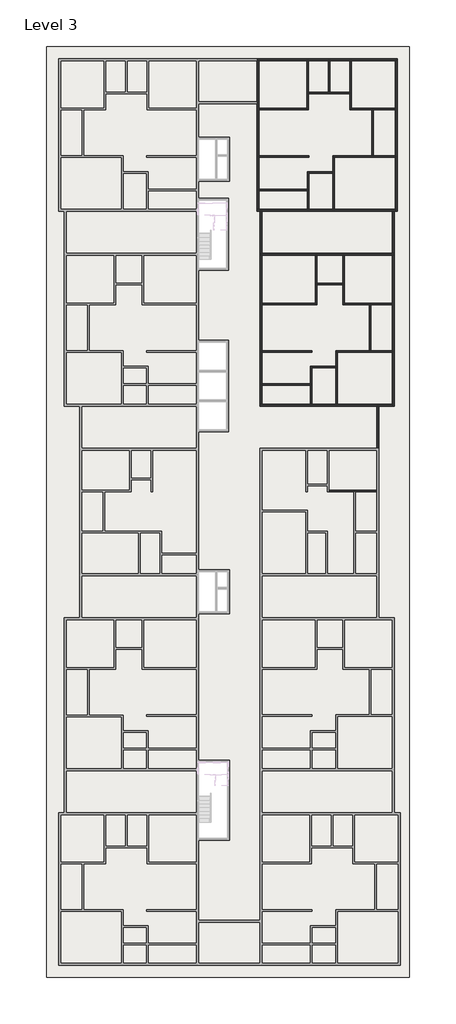
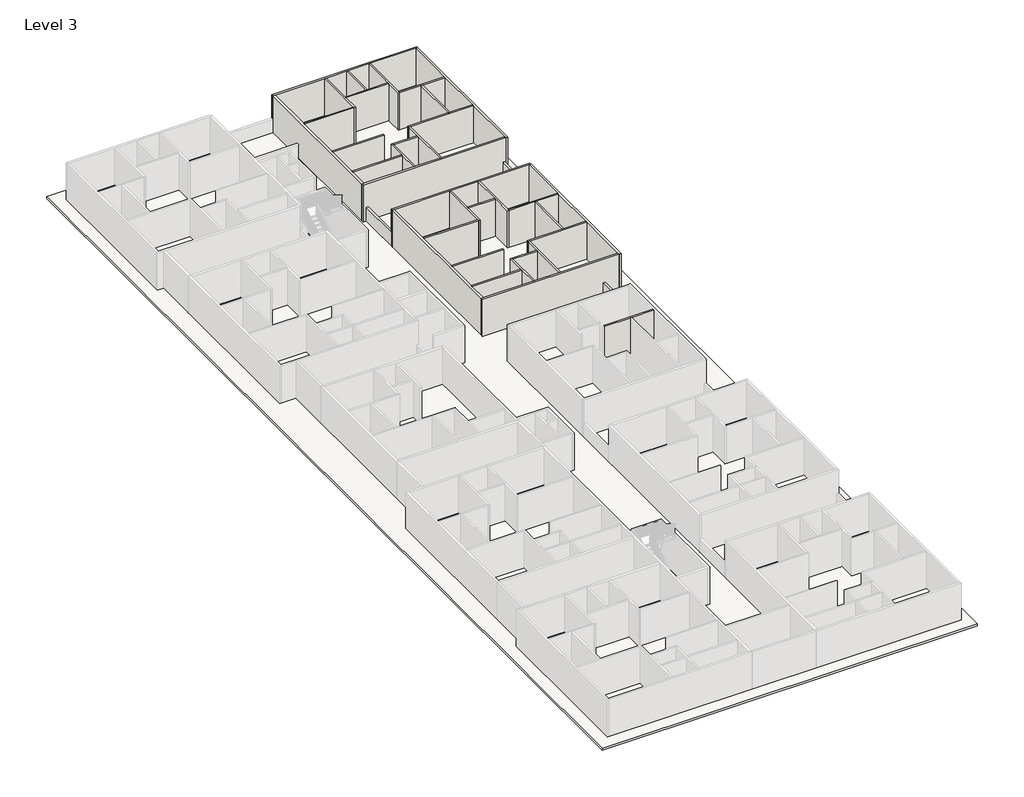
# One storey, part 4 of 8: 37 walls, 1 roof, 1 slab.
"""IFC4 building model written with IfcOpenShell, lengths in millimetres."""

from ifc_helpers import new_model, si_unit, frame, origin, place, context, project, spatial, polyline, outline, extrude, faceted_brep, element, save

model = new_model("IFC4")

# Units and contexts
model_context = context("Model", 3, world=origin())
ifc_project = project(units=[si_unit("LENGTHUNIT", "METRE", prefix="MILLI")], contexts=[model_context])

# Site, building, storey
site = spatial("IfcSite", under=ifc_project)
building = spatial("IfcBuilding", under=site)
storey = spatial("IfcBuildingStorey", under=building, Name="Level 3", Elevation=31330.6172466)

# Roof
placement = place(None, origin())
element("IfcRoof", 1, ObjectType="SLAB", at=placement, inside=storey, context=model_context, shape_type="SweptSolid", body=[
    extrude(outline(polyline([(-15237.9415084, -35021.5344126), (-15237.9415084, 36097.9216096), (12498.9443719, 36097.9216096), (12498.9443719, -35021.5344126), (-15237.9415084, -35021.5344126)]), holes=[polyline([(-3617.4415084, 29152.4900967), (-3617.4415084, 25799.6900967), (-1255.2415084, 25799.6900967), (-1255.2415084, 29152.4900967), (-3617.4415084, 29152.4900967)]), polyline([(-3617.4415084, 24490.1216096), (-3617.4415084, 19003.7216096), (-1331.4415084, 19003.7216096), (-1331.4415084, 24490.1216096), (-3617.4415084, 24490.1216096)]), polyline([(-3617.4415084, 13669.6303368), (-3617.4415084, 6659.2303368), (-1331.4415084, 6659.2303368), (-1331.4415084, 13669.6303368), (-3617.4415084, 13669.6303368)]), polyline([(-3617.4415084, -3882.2751812), (-3617.4415084, -7235.0751812), (-1255.2415084, -7235.0751812), (-1255.2415084, -3882.2751812), (-3617.4415084, -3882.2751812)]), polyline([(-3617.4415084, -18429.9851539), (-3617.4415084, -24525.9851539), (-1229.8415084, -24525.9851539), (-1229.8415084, -18429.9851539), (-3617.4415084, -18429.9851539)])]), frame((0.0, 0.0, 31330.6172466), z_axis=(0.0, 0.0, 1.0), x_axis=(1.0, 0.0, 0.0)), (0.0, 0.0, 1.0), 152.4),
])

# Slab
element("IfcSlab", 2, ObjectType="FLOOR", at=placement, inside=storey, context=model_context, shape_type="SweptSolid", body=[
    extrude(outline(polyline([(-14323.5415084, 35183.5216096), (11584.5443719, 35183.5216096), (11584.5443719, 23499.5216096), (11360.9214687, 23499.5216096), (11360.9214687, 8615.1216096), (10173.4714687, 8615.1216096), (10173.4714687, -7538.7344126), (11360.9214687, -7538.7344126), (11360.9214687, -22423.1344126), (11813.0584916, -22423.1344126), (11813.0584916, -34107.1344126), (11584.5443719, -34107.1344126), (-14323.5415084, -34107.1344126), (-14323.5415084, 35183.5216096)]), holes=[polyline([(-3617.4415084, 29152.4900967), (-3617.4415084, 25799.6900967), (-1255.2415084, 25799.6900967), (-1255.2415084, 29152.4900967), (-3617.4415084, 29152.4900967)]), polyline([(-3617.4415084, 24490.1216096), (-3617.4415084, 19003.7216096), (-1331.4415084, 19003.7216096), (-1331.4415084, 24490.1216096), (-3617.4415084, 24490.1216096)]), polyline([(-3617.4415084, 13669.6303368), (-3617.4415084, 6659.2303368), (-1331.4415084, 6659.2303368), (-1331.4415084, 13669.6303368), (-3617.4415084, 13669.6303368)]), polyline([(-3617.4415084, -3882.2751812), (-3617.4415084, -7235.0751812), (-1255.2415084, -7235.0751812), (-1255.2415084, -3882.2751812), (-3617.4415084, -3882.2751812)]), polyline([(-3617.4415084, -18429.9851539), (-3617.4415084, -24525.9851539), (-1229.8415084, -24525.9851539), (-1229.8415084, -18429.9851539), (-3617.4415084, -18429.9851539)])]), frame((0.0, 0.0, 30721.0172466), z_axis=(0.0, 0.0, 1.0), x_axis=(1.0, 0.0, 0.0)), (0.0, 0.0, 1.0), 609.6),
])

# Walls
element("IfcWall", 3, ObjectType="4.5\"", at=placement, inside=storey, context=model_context, shape_type="Brep", body=[
    faceted_brep([(6363.4714687, 2100.0216096, 31330.6172466), (8282.4584916, 2100.0216096, 31330.6172466), (8396.7584916, 2100.0216096, 31330.6172466), (10021.0714687, 2100.0216096, 31330.6172466), (10021.0714687, 2100.0216096, 34378.6172466), (8396.7584916, 2100.0216096, 34378.6172466), (8282.4584916, 2100.0216096, 34378.6172466), (6363.4714687, 2100.0216096, 34378.6172466), (6363.4714687, 2214.3216096, 31330.6172466), (6363.4714687, 2214.3216096, 34378.6172466), (10021.0714687, 2214.3216096, 34378.6172466), (10021.0714687, 2214.3216096, 31330.6172466)], [[[0, 1, 2, 3, 4, 5, 6, 7]], [[8, 9, 10, 11]], [[3, 2, 1, 0, 8, 11]], [[0, 7, 9, 8]], [[4, 3, 11, 10]], [[7, 6, 5, 4, 10, 9]]]),
])
element("IfcWall", 4, ObjectType="4.5\"", at=placement, inside=storey, context=model_context, shape_type="Brep", body=[
    faceted_brep([(5315.7214687, 20146.7216096, 31330.6172466), (5315.7214687, 16489.1216096, 31330.6172466), (5315.7214687, 16374.8216096, 31330.6172466), (5315.7214687, 16374.8216096, 34378.6172466), (5315.7214687, 16489.1216096, 34378.6172466), (5315.7214687, 20146.7216096, 34378.6172466), (5430.0214687, 20146.7216096, 31330.6172466), (5430.0214687, 20146.7216096, 34378.6172466), (5430.0214687, 18013.1216096, 34378.6172466), (5430.0214687, 17898.8216096, 34378.6172466), (5430.0214687, 16374.8216096, 34378.6172466), (5430.0214687, 16374.8216096, 31330.6172466), (5430.0214687, 17898.8216096, 31330.6172466), (5430.0214687, 18013.1216096, 31330.6172466)], [[[0, 1, 2, 3, 4, 5]], [[6, 7, 8, 9, 10, 11, 12, 13]], [[2, 1, 0, 6, 13, 12, 11]], [[0, 5, 7, 6]], [[3, 2, 11, 10]], [[5, 4, 3, 10, 9, 8, 7]]]),
])
element("IfcWall", 5, ObjectType="4.5\"", at=placement, inside=storey, context=model_context, shape_type="SweptSolid", body=[
    extrude(outline(polyline([(1259.3584916, 16489.1216096), (5315.7214687, 16489.1216096), (5315.7214687, 16374.8216096), (1259.3584916, 16374.8216096), (1259.3584916, 16489.1216096)])), frame((0.0, 0.0, 31330.6172466), z_axis=(0.0, 0.0, 1.0), x_axis=(1.0, 0.0, 0.0)), (0.0, 0.0, 1.0), 3048.0),
])
element("IfcWall", 6, ObjectType="4.5\"", at=placement, inside=storey, context=model_context, shape_type="SweptSolid", body=[
    extrude(outline(polyline([(7436.6214687, 17898.8216096), (5430.0214687, 17898.8216096), (5430.0214687, 18013.1216096), (7436.6214687, 18013.1216096), (7436.6214687, 17898.8216096)])), frame((0.0, 0.0, 31330.6172466), z_axis=(0.0, 0.0, 1.0), x_axis=(1.0, 0.0, 0.0)), (0.0, 0.0, 1.0), 3048.0),
])
element("IfcWall", 7, ObjectType="4.5\"", at=placement, inside=storey, context=model_context, shape_type="Brep", body=[
    faceted_brep([(7436.6214687, 20146.7216096, 31330.6172466), (7436.6214687, 18013.1216096, 31330.6172466), (7436.6214687, 17898.8216096, 31330.6172466), (7436.6214687, 16374.8216096, 31330.6172466), (7436.6214687, 16374.8216096, 34378.6172466), (7436.6214687, 17898.8216096, 34378.6172466), (7436.6214687, 18013.1216096, 34378.6172466), (7436.6214687, 20146.7216096, 34378.6172466), (7550.9214687, 20146.7216096, 31330.6172466), (7550.9214687, 20146.7216096, 34378.6172466), (7550.9214687, 16489.1216096, 34378.6172466), (7550.9214687, 16374.8216096, 34378.6172466), (7550.9214687, 16374.8216096, 31330.6172466), (7550.9214687, 16489.1216096, 31330.6172466)], [[[0, 1, 2, 3, 4, 5, 6, 7]], [[8, 9, 10, 11, 12, 13]], [[3, 2, 1, 0, 8, 13, 12]], [[0, 7, 9, 8]], [[4, 3, 12, 11]], [[7, 6, 5, 4, 11, 10, 9]]]),
])
element("IfcWall", 8, ObjectType="4.5\"", at=placement, inside=storey, context=model_context, shape_type="Brep", body=[
    faceted_brep([(7550.9214687, 16374.8216096, 31330.6172466), (9469.9084916, 16374.8216096, 31330.6172466), (9584.2084916, 16374.8216096, 31330.6172466), (11208.5214687, 16374.8216096, 31330.6172466), (11208.5214687, 16374.8216096, 34378.6172466), (9584.2084916, 16374.8216096, 34378.6172466), (9469.9084916, 16374.8216096, 34378.6172466), (7550.9214687, 16374.8216096, 34378.6172466), (7550.9214687, 16489.1216096, 31330.6172466), (7550.9214687, 16489.1216096, 34378.6172466), (11208.5214687, 16489.1216096, 34378.6172466), (11208.5214687, 16489.1216096, 31330.6172466)], [[[0, 1, 2, 3, 4, 5, 6, 7]], [[8, 9, 10, 11]], [[3, 2, 1, 0, 8, 11]], [[0, 7, 9, 8]], [[4, 3, 11, 10]], [[7, 6, 5, 4, 10, 9]]]),
])
element("IfcWall", 9, ObjectType="4.5\"", at=placement, inside=storey, context=model_context, shape_type="SweptSolid", body=[
    extrude(outline(polyline([(9469.9084916, 12869.6216096), (9469.9084916, 16374.8216096), (9584.2084916, 16374.8216096), (9584.2084916, 12869.6216096), (9469.9084916, 12869.6216096)])), frame((0.0, 0.0, 31330.6172466), z_axis=(0.0, 0.0, 1.0), x_axis=(1.0, 0.0, 0.0)), (0.0, 0.0, 1.0), 3048.0),
])
element("IfcWall", 10, ObjectType="4.5\"", at=placement, inside=storey, context=model_context, shape_type="Brep", body=[
    faceted_brep([(11208.5214687, 12869.6216096, 31330.6172466), (9584.2084916, 12869.6216096, 31330.6172466), (9469.9084916, 12869.6216096, 31330.6172466), (6885.4584916, 12869.6216096, 31330.6172466), (6885.4584916, 12869.6216096, 34378.6172466), (9469.9084916, 12869.6216096, 34378.6172466), (9584.2084916, 12869.6216096, 34378.6172466), (11208.5214687, 12869.6216096, 34378.6172466), (11208.5214687, 12755.3216096, 31330.6172466), (11208.5214687, 12755.3216096, 34378.6172466), (6999.7584916, 12755.3216096, 34378.6172466), (6885.4584916, 12755.3216096, 34378.6172466), (6885.4584916, 12755.3216096, 31330.6172466), (6999.7584916, 12755.3216096, 31330.6172466)], [[[0, 1, 2, 3, 4, 5, 6, 7]], [[8, 9, 10, 11, 12, 13]], [[3, 2, 1, 0, 8, 13, 12]], [[0, 7, 9, 8]], [[4, 3, 12, 11]], [[7, 6, 5, 4, 11, 10, 9]]]),
])
element("IfcWall", 11, ObjectType="4.5\"", at=placement, inside=storey, context=model_context, shape_type="Brep", body=[
    faceted_brep([(6885.4584916, 12755.3216096, 31330.6172466), (6885.4584916, 11663.1216096, 31330.6172466), (6885.4584916, 11548.8216096, 31330.6172466), (6885.4584916, 8767.5216096, 31330.6172466), (6885.4584916, 8767.5216096, 34378.6172466), (6885.4584916, 11548.8216096, 34378.6172466), (6885.4584916, 11663.1216096, 34378.6172466), (6885.4584916, 12755.3216096, 34378.6172466), (6999.7584916, 12755.3216096, 31330.6172466), (6999.7584916, 12755.3216096, 34378.6172466), (6999.7584916, 8767.5216096, 34378.6172466), (6999.7584916, 8767.5216096, 31330.6172466)], [[[0, 1, 2, 3, 4, 5, 6, 7]], [[8, 9, 10, 11]], [[3, 2, 1, 0, 8, 11]], [[0, 7, 9, 8]], [[4, 3, 11, 10]], [[7, 6, 5, 4, 10, 9]]]),
])
element("IfcWall", 12, ObjectType="4.5\"", at=placement, inside=storey, context=model_context, shape_type="Brep", body=[
    faceted_brep([(5056.6584916, 8767.5216096, 31330.6172466), (5056.6584916, 11548.8216096, 31330.6172466), (5056.6584916, 11663.1216096, 31330.6172466), (5056.6584916, 11663.1216096, 34378.6172466), (5056.6584916, 11548.8216096, 34378.6172466), (5056.6584916, 8767.5216096, 34378.6172466), (4942.3584916, 8767.5216096, 31330.6172466), (4942.3584916, 8767.5216096, 34378.6172466), (4942.3584916, 10215.3216096, 34378.6172466), (4942.3584916, 10329.6216096, 34378.6172466), (4942.3584916, 11663.1216096, 34378.6172466), (4942.3584916, 11663.1216096, 31330.6172466), (4942.3584916, 10329.6216096, 31330.6172466), (4942.3584916, 10215.3216096, 31330.6172466)], [[[0, 1, 2, 3, 4, 5]], [[6, 7, 8, 9, 10, 11, 12, 13]], [[2, 1, 0, 6, 13, 12, 11]], [[0, 5, 7, 6]], [[3, 2, 11, 10]], [[5, 4, 3, 10, 9, 8, 7]]]),
])
element("IfcWall", 13, ObjectType="4.5\"", at=placement, inside=storey, context=model_context, shape_type="SweptSolid", body=[
    extrude(outline(polyline([(6885.4584916, 11548.8216096), (5056.6584916, 11548.8216096), (5056.6584916, 11663.1216096), (6885.4584916, 11663.1216096), (6885.4584916, 11548.8216096)])), frame((0.0, 0.0, 31330.6172466), z_axis=(0.0, 0.0, 1.0), x_axis=(1.0, 0.0, 0.0)), (0.0, 0.0, 1.0), 3048.0),
])
element("IfcWall", 14, ObjectType="4.5\"", at=placement, inside=storey, context=model_context, shape_type="SweptSolid", body=[
    extrude(outline(polyline([(4942.3584916, 10215.3216096), (1259.3584916, 10215.3216096), (1259.3584916, 10329.6216096), (4942.3584916, 10329.6216096), (4942.3584916, 10215.3216096)])), frame((0.0, 0.0, 31330.6172466), z_axis=(0.0, 0.0, 1.0), x_axis=(1.0, 0.0, 0.0)), (0.0, 0.0, 1.0), 3048.0),
])
element("IfcWall", 15, ObjectType="4.5\"", at=placement, inside=storey, context=model_context, shape_type="SweptSolid", body=[
    extrude(outline(polyline([(5056.6584916, 12755.3216096), (1259.3584916, 12755.3216096), (1259.3584916, 12869.6216096), (5056.6584916, 12869.6216096), (5056.6584916, 12755.3216096)])), frame((0.0, 0.0, 31330.6172466), z_axis=(0.0, 0.0, 1.0), x_axis=(1.0, 0.0, 0.0)), (0.0, 0.0, 1.0), 3048.0),
])
element("IfcWall", 16, ObjectType="4.5\"", at=placement, inside=storey, context=model_context, shape_type="Brep", body=[
    faceted_brep([(4688.4443719, 35031.1216096, 31330.6172466), (4688.4443719, 31373.5216096, 31330.6172466), (4688.4443719, 31259.2216096, 31330.6172466), (4688.4443719, 31259.2216096, 34378.6172466), (4688.4443719, 31373.5216096, 34378.6172466), (4688.4443719, 35031.1216096, 34378.6172466), (4802.7443719, 35031.1216096, 31330.6172466), (4802.7443719, 35031.1216096, 34378.6172466), (4802.7443719, 32592.7216096, 34378.6172466), (4802.7443719, 32478.4216096, 34378.6172466), (4802.7443719, 31259.2216096, 34378.6172466), (4802.7443719, 31259.2216096, 31330.6172466), (4802.7443719, 32478.4216096, 31330.6172466), (4802.7443719, 32592.7216096, 31330.6172466)], [[[0, 1, 2, 3, 4, 5]], [[6, 7, 8, 9, 10, 11, 12, 13]], [[2, 1, 0, 6, 13, 12, 11]], [[0, 5, 7, 6]], [[3, 2, 11, 10]], [[5, 4, 3, 10, 9, 8, 7]]]),
])
element("IfcWall", 17, ObjectType="4.5\"", at=placement, inside=storey, context=model_context, shape_type="SweptSolid", body=[
    extrude(outline(polyline([(1030.8443719, 31373.5216096), (4688.4443719, 31373.5216096), (4688.4443719, 31259.2216096), (1030.8443719, 31259.2216096), (1030.8443719, 31373.5216096)])), frame((0.0, 0.0, 31330.6172466), z_axis=(0.0, 0.0, 1.0), x_axis=(1.0, 0.0, 0.0)), (0.0, 0.0, 1.0), 3048.0),
])
element("IfcWall", 18, ObjectType="4.5\"", at=placement, inside=storey, context=model_context, shape_type="Brep", body=[
    faceted_brep([(4802.7443719, 32478.4216096, 31330.6172466), (7965.0443719, 32478.4216096, 31330.6172466), (7965.0443719, 32478.4216096, 34378.6172466), (4802.7443719, 32478.4216096, 34378.6172466), (4802.7443719, 32592.7216096, 31330.6172466), (4802.7443719, 32592.7216096, 34378.6172466), (6326.7443719, 32592.7216096, 34378.6172466), (6441.0443719, 32592.7216096, 34378.6172466), (7965.0443719, 32592.7216096, 34378.6172466), (7965.0443719, 32592.7216096, 31330.6172466), (6441.0443719, 32592.7216096, 31330.6172466), (6326.7443719, 32592.7216096, 31330.6172466)], [[[0, 1, 2, 3]], [[4, 5, 6, 7, 8, 9, 10, 11]], [[1, 0, 4, 11, 10, 9]], [[0, 3, 5, 4]], [[2, 1, 9, 8]], [[3, 2, 8, 7, 6, 5]]]),
])
element("IfcWall", 19, ObjectType="4.5\"", at=placement, inside=storey, context=model_context, shape_type="SweptSolid", body=[
    extrude(outline(polyline([(6326.7443719, 32592.7216096), (6326.7443719, 35031.1216096), (6441.0443719, 35031.1216096), (6441.0443719, 32592.7216096), (6326.7443719, 32592.7216096)])), frame((0.0, 0.0, 31330.6172466), z_axis=(0.0, 0.0, 1.0), x_axis=(1.0, 0.0, 0.0)), (0.0, 0.0, 1.0), 3048.0),
])
element("IfcWall", 20, ObjectType="4.5\"", at=placement, inside=storey, context=model_context, shape_type="Brep", body=[
    faceted_brep([(7965.0443719, 35031.1216096, 31330.6172466), (7965.0443719, 32592.7216096, 31330.6172466), (7965.0443719, 32478.4216096, 31330.6172466), (7965.0443719, 31259.2216096, 31330.6172466), (7965.0443719, 31259.2216096, 34378.6172466), (7965.0443719, 32478.4216096, 34378.6172466), (7965.0443719, 32592.7216096, 34378.6172466), (7965.0443719, 35031.1216096, 34378.6172466), (8079.3443719, 35031.1216096, 31330.6172466), (8079.3443719, 35031.1216096, 34378.6172466), (8079.3443719, 31373.5216096, 34378.6172466), (8079.3443719, 31259.2216096, 34378.6172466), (8079.3443719, 31259.2216096, 31330.6172466), (8079.3443719, 31373.5216096, 31330.6172466)], [[[0, 1, 2, 3, 4, 5, 6, 7]], [[8, 9, 10, 11, 12, 13]], [[3, 2, 1, 0, 8, 13, 12]], [[0, 7, 9, 8]], [[4, 3, 12, 11]], [[7, 6, 5, 4, 11, 10, 9]]]),
])
element("IfcWall", 21, ObjectType="4.5\"", at=placement, inside=storey, context=model_context, shape_type="Brep", body=[
    faceted_brep([(8079.3443719, 31259.2216096, 31330.6172466), (9641.4443719, 31259.2216096, 31330.6172466), (9755.7443719, 31259.2216096, 31330.6172466), (11432.1443719, 31259.2216096, 31330.6172466), (11432.1443719, 31259.2216096, 34378.6172466), (9755.7443719, 31259.2216096, 34378.6172466), (9641.4443719, 31259.2216096, 34378.6172466), (8079.3443719, 31259.2216096, 34378.6172466), (8079.3443719, 31373.5216096, 31330.6172466), (8079.3443719, 31373.5216096, 34378.6172466), (11432.1443719, 31373.5216096, 34378.6172466), (11432.1443719, 31373.5216096, 31330.6172466)], [[[0, 1, 2, 3, 4, 5, 6, 7]], [[8, 9, 10, 11]], [[3, 2, 1, 0, 8, 11]], [[0, 7, 9, 8]], [[4, 3, 11, 10]], [[7, 6, 5, 4, 10, 9]]]),
])
element("IfcWall", 22, ObjectType="4.5\"", at=placement, inside=storey, context=model_context, shape_type="SweptSolid", body=[
    extrude(outline(polyline([(9641.4443719, 27754.0216096), (9641.4443719, 31259.2216096), (9755.7443719, 31259.2216096), (9755.7443719, 27754.0216096), (9641.4443719, 27754.0216096)])), frame((0.0, 0.0, 31330.6172466), z_axis=(0.0, 0.0, 1.0), x_axis=(1.0, 0.0, 0.0)), (0.0, 0.0, 1.0), 3048.0),
])
element("IfcWall", 23, ObjectType="4.5\"", at=placement, inside=storey, context=model_context, shape_type="Brep", body=[
    faceted_brep([(11432.1443719, 27754.0216096, 31330.6172466), (9755.7443719, 27754.0216096, 31330.6172466), (9641.4443719, 27754.0216096, 31330.6172466), (6656.9443719, 27754.0216096, 31330.6172466), (6656.9443719, 27754.0216096, 34378.6172466), (9641.4443719, 27754.0216096, 34378.6172466), (9755.7443719, 27754.0216096, 34378.6172466), (11432.1443719, 27754.0216096, 34378.6172466), (11432.1443719, 27639.7216096, 31330.6172466), (11432.1443719, 27639.7216096, 34378.6172466), (6771.2443719, 27639.7216096, 34378.6172466), (6656.9443719, 27639.7216096, 34378.6172466), (6656.9443719, 27639.7216096, 31330.6172466), (6771.2443719, 27639.7216096, 31330.6172466)], [[[0, 1, 2, 3, 4, 5, 6, 7]], [[8, 9, 10, 11, 12, 13]], [[3, 2, 1, 0, 8, 13, 12]], [[0, 7, 9, 8]], [[4, 3, 12, 11]], [[7, 6, 5, 4, 11, 10, 9]]]),
])
element("IfcWall", 24, ObjectType="4.5\"", at=placement, inside=storey, context=model_context, shape_type="Brep", body=[
    faceted_brep([(6656.9443719, 27639.7216096, 31330.6172466), (6656.9443719, 26547.5216096, 31330.6172466), (6656.9443719, 26433.2216096, 31330.6172466), (6656.9443719, 23651.9216096, 31330.6172466), (6656.9443719, 23651.9216096, 34378.6172466), (6656.9443719, 26433.2216096, 34378.6172466), (6656.9443719, 26547.5216096, 34378.6172466), (6656.9443719, 27639.7216096, 34378.6172466), (6771.2443719, 27639.7216096, 31330.6172466), (6771.2443719, 27639.7216096, 34378.6172466), (6771.2443719, 23651.9216096, 34378.6172466), (6771.2443719, 23651.9216096, 31330.6172466)], [[[0, 1, 2, 3, 4, 5, 6, 7]], [[8, 9, 10, 11]], [[3, 2, 1, 0, 8, 11]], [[0, 7, 9, 8]], [[4, 3, 11, 10]], [[7, 6, 5, 4, 10, 9]]]),
])
element("IfcWall", 25, ObjectType="4.5\"", at=placement, inside=storey, context=model_context, shape_type="SweptSolid", body=[
    extrude(outline(polyline([(4713.8443719, 25099.7216096), (1030.8443719, 25099.7216096), (1030.8443719, 25214.0216096), (4713.8443719, 25214.0216096), (4713.8443719, 25099.7216096)])), frame((0.0, 0.0, 31330.6172466), z_axis=(0.0, 0.0, 1.0), x_axis=(1.0, 0.0, 0.0)), (0.0, 0.0, 1.0), 3048.0),
])
element("IfcWall", 26, ObjectType="4.5\"", at=placement, inside=storey, context=model_context, shape_type="Brep", body=[
    faceted_brep([(4828.1443719, 23651.9216096, 31330.6172466), (4828.1443719, 26433.2216096, 31330.6172466), (4828.1443719, 26547.5216096, 31330.6172466), (4828.1443719, 26547.5216096, 34378.6172466), (4828.1443719, 26433.2216096, 34378.6172466), (4828.1443719, 23651.9216096, 34378.6172466), (4713.8443719, 23651.9216096, 31330.6172466), (4713.8443719, 23651.9216096, 34378.6172466), (4713.8443719, 25099.7216096, 34378.6172466), (4713.8443719, 25214.0216096, 34378.6172466), (4713.8443719, 26547.5216096, 34378.6172466), (4713.8443719, 26547.5216096, 31330.6172466), (4713.8443719, 25214.0216096, 31330.6172466), (4713.8443719, 25099.7216096, 31330.6172466)], [[[0, 1, 2, 3, 4, 5]], [[6, 7, 8, 9, 10, 11, 12, 13]], [[2, 1, 0, 6, 13, 12, 11]], [[0, 5, 7, 6]], [[3, 2, 11, 10]], [[5, 4, 3, 10, 9, 8, 7]]]),
])
element("IfcWall", 27, ObjectType="4.5\"", at=placement, inside=storey, context=model_context, shape_type="SweptSolid", body=[
    extrude(outline(polyline([(6656.9443719, 26433.2216096), (4828.1443719, 26433.2216096), (4828.1443719, 26547.5216096), (6656.9443719, 26547.5216096), (6656.9443719, 26433.2216096)])), frame((0.0, 0.0, 31330.6172466), z_axis=(0.0, 0.0, 1.0), x_axis=(1.0, 0.0, 0.0)), (0.0, 0.0, 1.0), 3048.0),
])
element("IfcWall", 28, ObjectType="4.5\"", at=placement, inside=storey, context=model_context, shape_type="SweptSolid", body=[
    extrude(outline(polyline([(4828.1443719, 27639.7216096), (1030.8443719, 27639.7216096), (1030.8443719, 27754.0216096), (4828.1443719, 27754.0216096), (4828.1443719, 27639.7216096)])), frame((0.0, 0.0, 31330.6172466), z_axis=(0.0, 0.0, 1.0), x_axis=(1.0, 0.0, 0.0)), (0.0, 0.0, 1.0), 3048.0),
])
element("IfcWall", 29, ObjectType="6\"", at=placement, inside=storey, context=model_context, shape_type="Brep", body=[
    faceted_brep([(1106.9584916, 20146.7216096, 34378.6172466), (1106.9584916, 20146.7216096, 31330.6172466), (1259.3584916, 20146.7216096, 31330.6172466), (5315.7214687, 20146.7216096, 31330.6172466), (5430.0214687, 20146.7216096, 31330.6172466), (7436.6214687, 20146.7216096, 31330.6172466), (7550.9214687, 20146.7216096, 31330.6172466), (11208.5214687, 20146.7216096, 31330.6172466), (11360.9214687, 20146.7216096, 31330.6172466), (11360.9214687, 20146.7216096, 34378.6172466), (11208.5214687, 20146.7216096, 34378.6172466), (7550.9214687, 20146.7216096, 34378.6172466), (7436.6214687, 20146.7216096, 34378.6172466), (5430.0214687, 20146.7216096, 34378.6172466), (5315.7214687, 20146.7216096, 34378.6172466), (1259.3584916, 20146.7216096, 34378.6172466), (1106.9584916, 20299.1216096, 31330.6172466), (1106.9584916, 20299.1216096, 32549.8172466), (1106.9584916, 20299.1216096, 34378.6172466), (11360.9214687, 20299.1216096, 34378.6172466), (11360.9214687, 20299.1216096, 32549.8172466), (11360.9214687, 20299.1216096, 31330.6172466), (11208.5214687, 20299.1216096, 31330.6172466), (1259.3584916, 20299.1216096, 31330.6172466)], [[[0, 1, 2, 3, 4, 5, 6, 7, 8, 9, 10, 11, 12, 13, 14, 15]], [[16, 17, 18, 19, 20, 21, 22, 23]], [[8, 7, 6, 5, 4, 3, 2, 1, 16, 23, 22, 21]], [[0, 18, 17, 16, 1]], [[8, 21, 20, 19, 9]], [[0, 15, 14, 13, 12, 11, 10, 9, 19, 18]]]),
])
element("IfcWall", 30, ObjectType="6\"", at=placement, inside=storey, context=model_context, shape_type="Brep", body=[
    faceted_brep([(11208.5214687, 20146.7216096, 34378.6172466), (11208.5214687, 20146.7216096, 31330.6172466), (11208.5214687, 16489.1216096, 31330.6172466), (11208.5214687, 16374.8216096, 31330.6172466), (11208.5214687, 12869.6216096, 31330.6172466), (11208.5214687, 12755.3216096, 31330.6172466), (11208.5214687, 8767.5216096, 31330.6172466), (11208.5214687, 8615.1216096, 31330.6172466), (11208.5214687, 8615.1216096, 34378.6172466), (11208.5214687, 8767.5216096, 34378.6172466), (11208.5214687, 12755.3216096, 34378.6172466), (11208.5214687, 12869.6216096, 34378.6172466), (11208.5214687, 16374.8216096, 34378.6172466), (11208.5214687, 16489.1216096, 34378.6172466), (11360.9214687, 20146.7216096, 31330.6172466), (11360.9214687, 20146.7216096, 34378.6172466), (11360.9214687, 8615.1216096, 34378.6172466), (11360.9214687, 8615.1216096, 31330.6172466)], [[[0, 1, 2, 3, 4, 5, 6, 7, 8, 9, 10, 11, 12, 13]], [[14, 15, 16, 17]], [[7, 6, 5, 4, 3, 2, 1, 14, 17]], [[8, 7, 17, 16]], [[0, 15, 14, 1]], [[0, 13, 12, 11, 10, 9, 8, 16, 15]]]),
])
element("IfcWall", 31, ObjectType="6\"", at=placement, inside=storey, context=model_context, shape_type="Brep", body=[
    faceted_brep([(11208.5214687, 8767.5216096, 31330.6172466), (6999.7584916, 8767.5216096, 31330.6172466), (6885.4584916, 8767.5216096, 31330.6172466), (5056.6584916, 8767.5216096, 31330.6172466), (4942.3584916, 8767.5216096, 31330.6172466), (1259.3584916, 8767.5216096, 31330.6172466), (1106.9584916, 8767.5216096, 31330.6172466), (1106.9584916, 8767.5216096, 34378.6172466), (1259.3584916, 8767.5216096, 34378.6172466), (4942.3584916, 8767.5216096, 34378.6172466), (5056.6584916, 8767.5216096, 34378.6172466), (6885.4584916, 8767.5216096, 34378.6172466), (6999.7584916, 8767.5216096, 34378.6172466), (11208.5214687, 8767.5216096, 34378.6172466), (11208.5214687, 8615.1216096, 31330.6172466), (11208.5214687, 8615.1216096, 34378.6172466), (1106.9584916, 8615.1216096, 34378.6172466), (1106.9584916, 8615.1216096, 31330.6172466), (10021.0714687, 8615.1216096, 31330.6172466), (10173.4714687, 8615.1216096, 31330.6172466)], [[[0, 1, 2, 3, 4, 5, 6, 7, 8, 9, 10, 11, 12, 13]], [[14, 15, 16, 17, 18, 19]], [[6, 5, 4, 3, 2, 1, 0, 14, 19, 18, 17]], [[0, 13, 15, 14]], [[7, 6, 17, 16]], [[13, 12, 11, 10, 9, 8, 7, 16, 15]]]),
])
element("IfcWall", 32, ObjectType="6\"", at=placement, inside=storey, context=model_context, shape_type="Brep", body=[
    faceted_brep([(1259.3584916, 8767.5216096, 31330.6172466), (1259.3584916, 10215.3216096, 31330.6172466), (1259.3584916, 10329.6216096, 31330.6172466), (1259.3584916, 12755.3216096, 31330.6172466), (1259.3584916, 12869.6216096, 31330.6172466), (1259.3584916, 16374.8216096, 31330.6172466), (1259.3584916, 16489.1216096, 31330.6172466), (1259.3584916, 20146.7216096, 31330.6172466), (1259.3584916, 20146.7216096, 34378.6172466), (1259.3584916, 16489.1216096, 34378.6172466), (1259.3584916, 16374.8216096, 34378.6172466), (1259.3584916, 12869.6216096, 34378.6172466), (1259.3584916, 12755.3216096, 34378.6172466), (1259.3584916, 10329.6216096, 34378.6172466), (1259.3584916, 10215.3216096, 34378.6172466), (1259.3584916, 8767.5216096, 34378.6172466), (1106.9584916, 8767.5216096, 31330.6172466), (1106.9584916, 8767.5216096, 34378.6172466), (1106.9584916, 20146.7216096, 34378.6172466), (1106.9584916, 20146.7216096, 31330.6172466)], [[[0, 1, 2, 3, 4, 5, 6, 7, 8, 9, 10, 11, 12, 13, 14, 15]], [[16, 17, 18, 19]], [[7, 6, 5, 4, 3, 2, 1, 0, 16, 19]], [[0, 15, 17, 16]], [[7, 19, 18, 8]], [[15, 14, 13, 12, 11, 10, 9, 8, 18, 17]]]),
])
element("IfcWall", 33, ObjectType="6\"", at=placement, inside=storey, context=model_context, shape_type="Brep", body=[
    faceted_brep([(878.4443719, 35031.1216096, 34378.6172466), (878.4443719, 35031.1216096, 31330.6172466), (1030.8443719, 35031.1216096, 31330.6172466), (4688.4443719, 35031.1216096, 31330.6172466), (4802.7443719, 35031.1216096, 31330.6172466), (6326.7443719, 35031.1216096, 31330.6172466), (6441.0443719, 35031.1216096, 31330.6172466), (7965.0443719, 35031.1216096, 31330.6172466), (8079.3443719, 35031.1216096, 31330.6172466), (11432.1443719, 35031.1216096, 31330.6172466), (11584.5443719, 35031.1216096, 31330.6172466), (11584.5443719, 35031.1216096, 34378.6172466), (11432.1443719, 35031.1216096, 34378.6172466), (8079.3443719, 35031.1216096, 34378.6172466), (7965.0443719, 35031.1216096, 34378.6172466), (6441.0443719, 35031.1216096, 34378.6172466), (6326.7443719, 35031.1216096, 34378.6172466), (4802.7443719, 35031.1216096, 34378.6172466), (4688.4443719, 35031.1216096, 34378.6172466), (1030.8443719, 35031.1216096, 34378.6172466), (878.4443719, 35183.5216096, 31330.6172466), (878.4443719, 35183.5216096, 34378.6172466), (11584.5443719, 35183.5216096, 34378.6172466), (11584.5443719, 35183.5216096, 31330.6172466)], [[[0, 1, 2, 3, 4, 5, 6, 7, 8, 9, 10, 11, 12, 13, 14, 15, 16, 17, 18, 19]], [[20, 21, 22, 23]], [[10, 9, 8, 7, 6, 5, 4, 3, 2, 1, 20, 23]], [[11, 10, 23, 22]], [[0, 21, 20, 1]], [[0, 19, 18, 17, 16, 15, 14, 13, 12, 11, 22, 21]]]),
])
element("IfcWall", 34, ObjectType="6\"", at=placement, inside=storey, context=model_context, shape_type="Brep", body=[
    faceted_brep([(11432.1443719, 35031.1216096, 31330.6172466), (11432.1443719, 31373.5216096, 31330.6172466), (11432.1443719, 31259.2216096, 31330.6172466), (11432.1443719, 27754.0216096, 31330.6172466), (11432.1443719, 27639.7216096, 31330.6172466), (11432.1443719, 23651.9216096, 31330.6172466), (11432.1443719, 23499.5216096, 31330.6172466), (11432.1443719, 23499.5216096, 34378.6172466), (11432.1443719, 23651.9216096, 34378.6172466), (11432.1443719, 27639.7216096, 34378.6172466), (11432.1443719, 27754.0216096, 34378.6172466), (11432.1443719, 31259.2216096, 34378.6172466), (11432.1443719, 31373.5216096, 34378.6172466), (11432.1443719, 35031.1216096, 34378.6172466), (11584.5443719, 35031.1216096, 31330.6172466), (11584.5443719, 35031.1216096, 34378.6172466), (11584.5443719, 23499.5216096, 34378.6172466), (11584.5443719, 23499.5216096, 31330.6172466)], [[[0, 1, 2, 3, 4, 5, 6, 7, 8, 9, 10, 11, 12, 13]], [[14, 15, 16, 17]], [[6, 5, 4, 3, 2, 1, 0, 14, 17]], [[0, 13, 15, 14]], [[7, 6, 17, 16]], [[13, 12, 11, 10, 9, 8, 7, 16, 15]]]),
])
element("IfcWall", 35, ObjectType="6\"", at=placement, inside=storey, context=model_context, shape_type="Brep", body=[
    faceted_brep([(11432.1443719, 23651.9216096, 31330.6172466), (6771.2443719, 23651.9216096, 31330.6172466), (6656.9443719, 23651.9216096, 31330.6172466), (4828.1443719, 23651.9216096, 31330.6172466), (4713.8443719, 23651.9216096, 31330.6172466), (1030.8443719, 23651.9216096, 31330.6172466), (878.4443719, 23651.9216096, 31330.6172466), (878.4443719, 23651.9216096, 34378.6172466), (1030.8443719, 23651.9216096, 34378.6172466), (4713.8443719, 23651.9216096, 34378.6172466), (4828.1443719, 23651.9216096, 34378.6172466), (6656.9443719, 23651.9216096, 34378.6172466), (6771.2443719, 23651.9216096, 34378.6172466), (11432.1443719, 23651.9216096, 34378.6172466), (11432.1443719, 23499.5216096, 31330.6172466), (11432.1443719, 23499.5216096, 34378.6172466), (878.4443719, 23499.5216096, 34378.6172466), (878.4443719, 23499.5216096, 31330.6172466), (1106.9584916, 23499.5216096, 31330.6172466), (1259.3584916, 23499.5216096, 31330.6172466), (11208.5214687, 23499.5216096, 31330.6172466), (11360.9214687, 23499.5216096, 31330.6172466)], [[[0, 1, 2, 3, 4, 5, 6, 7, 8, 9, 10, 11, 12, 13]], [[14, 15, 16, 17, 18, 19, 20, 21]], [[6, 5, 4, 3, 2, 1, 0, 14, 21, 20, 19, 18, 17]], [[0, 13, 15, 14]], [[7, 6, 17, 16]], [[13, 12, 11, 10, 9, 8, 7, 16, 15]]]),
])
element("IfcWall", 36, ObjectType="6\"", at=placement, inside=storey, context=model_context, shape_type="Brep", body=[
    faceted_brep([(1030.8443719, 23651.9216096, 31330.6172466), (1030.8443719, 25099.7216096, 31330.6172466), (1030.8443719, 25214.0216096, 31330.6172466), (1030.8443719, 27639.7216096, 31330.6172466), (1030.8443719, 27754.0216096, 31330.6172466), (1030.8443719, 31259.2216096, 31330.6172466), (1030.8443719, 31373.5216096, 31330.6172466), (1030.8443719, 35031.1216096, 31330.6172466), (1030.8443719, 35031.1216096, 34378.6172466), (1030.8443719, 31373.5216096, 34378.6172466), (1030.8443719, 31259.2216096, 34378.6172466), (1030.8443719, 27754.0216096, 34378.6172466), (1030.8443719, 27639.7216096, 34378.6172466), (1030.8443719, 25214.0216096, 34378.6172466), (1030.8443719, 25099.7216096, 34378.6172466), (1030.8443719, 23651.9216096, 34378.6172466), (878.4443719, 23651.9216096, 31330.6172466), (878.4443719, 23651.9216096, 34378.6172466), (878.4443719, 35031.1216096, 34378.6172466), (878.4443719, 35031.1216096, 31330.6172466), (878.4443719, 31897.3197155, 31330.6172466), (878.4443719, 31744.9197155, 31330.6172466)], [[[0, 1, 2, 3, 4, 5, 6, 7, 8, 9, 10, 11, 12, 13, 14, 15]], [[16, 17, 18, 19, 20, 21]], [[7, 6, 5, 4, 3, 2, 1, 0, 16, 21, 20, 19]], [[0, 15, 17, 16]], [[7, 19, 18, 8]], [[15, 14, 13, 12, 11, 10, 9, 8, 18, 17]]]),
])
element("IfcWall", 37, ObjectType="6\" 2", at=placement, inside=storey, context=model_context, shape_type="SweptSolid", body=[
    extrude(outline(polyline([(1106.9584916, 20299.1216096), (1106.9584916, 23499.5216096), (1259.3584916, 23499.5216096), (1259.3584916, 20299.1216096), (1106.9584916, 20299.1216096)])), frame((0.0, 0.0, 31330.6172466), z_axis=(0.0, 0.0, 1.0), x_axis=(1.0, 0.0, 0.0)), (0.0, 0.0, 1.0), 1219.2),
])
element("IfcWall", 38, ObjectType="6\" 2", at=placement, inside=storey, context=model_context, shape_type="SweptSolid", body=[
    extrude(outline(polyline([(11208.5214687, 20299.1216096), (11208.5214687, 23499.5216096), (11360.9214687, 23499.5216096), (11360.9214687, 20299.1216096), (11208.5214687, 20299.1216096)])), frame((0.0, 0.0, 31330.6172466), z_axis=(0.0, 0.0, 1.0), x_axis=(1.0, 0.0, 0.0)), (0.0, 0.0, 1.0), 1219.2),
])
element("IfcWall", 39, ObjectType="6\" 2", at=placement, inside=storey, context=model_context, shape_type="SweptSolid", body=[
    extrude(outline(polyline([(10021.0714687, 5414.7216096), (10021.0714687, 8615.1216096), (10173.4714687, 8615.1216096), (10173.4714687, 5414.7216096), (10021.0714687, 5414.7216096)])), frame((0.0, 0.0, 31330.6172466), z_axis=(0.0, 0.0, 1.0), x_axis=(1.0, 0.0, 0.0)), (0.0, 0.0, 1.0), 1219.2),
])

save(model, "model.ifc")

# Revit data of these elements
# Type "SLAB"
#   Assembly Code = "B1020"
#   Layers, outside or top first: 0' - 6" "Damp-proofing" (function 1)
# Type "FLOOR"
#   Assembly Code = "B1010"
#   Function = 0
#   Layers, outside or top first: 2' - 0" "Tile, Porcelain, 4in" (function 1)
# Type "4.5\""
#   Assembly Code = "B2010"
#   Layers, outside or top first: 0' - 4 1/2" "WALLS" (function 1)
# Type "6\""
#   Assembly Code = "B2010"
#   Layers, outside or top first: 0' - 6" "WALLS" (function 1)
# Type "6\" 2"
#   Assembly Code = "B2010"
#   Layers, outside or top first: 0' - 6" "4'" (function 1)
# Element 1 (IfcRoof, "SLAB")
#   built-in parameter 1001705 = 103.291 (stored number, unit not read)
#   built-in parameter 1001710 = 33615
#   Phase Created = New Construction
#   Materials on its faces: "Damp-proofing"
# Element 2 (IfcSlab, "FLOOR")
#   built-in parameter 1001955 = 3.14159 (stored number, unit not read)
#   Height Offset From Level = 0' - 0"
#   Phase Created = New Construction
#   Materials on its faces: "Tile, Porcelain, 4in"
# Elements 3, 4, 5, 6, 7, 8, 9, 10, 11, 12, 13, 14, 15, 16, 17, 18, 19, 20, 21, 22, 23, 24, 25, 26, 27, 28 (IfcWall, "4.5\"")
#   Top Offset = 0' - 0"
#   Base Offset = 0' - 0"
#   Unconnected Height = 10' - 0"
#   wall height = 10' - 0"
#   Phase Created = New Construction
#   Base Constraint = Level 3
#   Materials on its faces: "WALLS"
# Elements 29, 30, 31, 32, 33, 34, 35, 36 (IfcWall, "6\"")
#   Top Offset = 0' - 0"
#   Base Offset = 0' - 0"
#   Unconnected Height = 10' - 0"
#   wall height = 10' - 0"
#   Phase Created = New Construction
#   Base Constraint = Level 3
#   Materials on its faces: "WALLS"
# Elements 37, 38, 39 (IfcWall, "6\" 2")
#   Top Offset = 0' - 0"
#   Base Offset = 0' - 0"
#   Unconnected Height = 4' - 0"
#   wall height = 4' - 0"
#   Phase Created = New Construction
#   Base Constraint = Level 3
#   Materials on its faces: "4'"
# Materials
#   "Damp-proofing": class "Generic", colour RGB 127 127 127, transparency 0, Description = "Damp-proofing", Cost = 0
#   "Tile, Porcelain, 4in": class "Generic", colour RGB 89 87 158, transparency 0, Description = "Porcelain tile, 4\", white", Cost = 0
#   "WALLS": class "Generic", colour RGB 120 120 120, transparency 0, Cost = 0
#   "4'": class "Generic", colour RGB 120 120 120, transparency 0, Cost = 0
